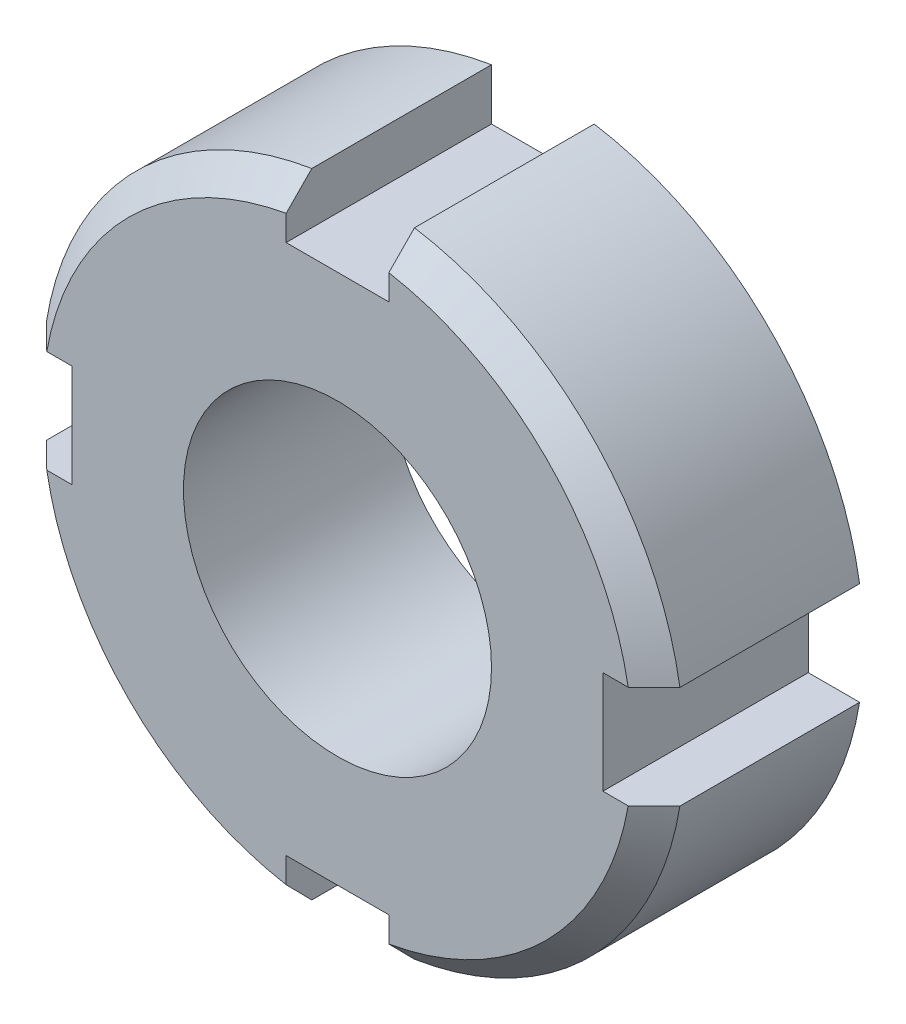
ISO-10303-21;
HEADER;
FILE_DESCRIPTION(('STEP AP214'),'2;1');
FILE_NAME('part.step','',(''),(''),'','','');
FILE_SCHEMA(('AUTOMOTIVE_DESIGN { 1 0 10303 214 1 1 1 1 }'));
ENDSEC;
DATA;
#1=APPLICATION_CONTEXT('core data for automotive mechanical design processes');
#2=APPLICATION_PROTOCOL_DEFINITION('international standard','automotive_design',2000,#1);
#3=PRODUCT_CONTEXT('',#1,'mechanical');
#4=PRODUCT('Part','Part','',(#3));
#5=PRODUCT_RELATED_PRODUCT_CATEGORY('part','',(#4));
#6=PRODUCT_DEFINITION_FORMATION('','',#4);
#7=PRODUCT_DEFINITION_CONTEXT('part definition',#1,'design');
#8=PRODUCT_DEFINITION('design','',#6,#7);
#9=PRODUCT_DEFINITION_SHAPE('','',#8);
#10=(LENGTH_UNIT() NAMED_UNIT(*) SI_UNIT(.MILLI.,.METRE.));
#11=(NAMED_UNIT(*) PLANE_ANGLE_UNIT() SI_UNIT($,.RADIAN.));
#12=(NAMED_UNIT(*) SI_UNIT($,.STERADIAN.) SOLID_ANGLE_UNIT());
#13=UNCERTAINTY_MEASURE_WITH_UNIT(LENGTH_MEASURE(1.E-05),#10,'distance_accuracy_value','');
#14=(GEOMETRIC_REPRESENTATION_CONTEXT(3) GLOBAL_UNCERTAINTY_ASSIGNED_CONTEXT((#13)) GLOBAL_UNIT_ASSIGNED_CONTEXT((#10,
#11,#12)) REPRESENTATION_CONTEXT('',''));
#15=CARTESIAN_POINT('',(0.,0.,0.));
#16=DIRECTION('',(0.,0.,1.));
#17=DIRECTION('',(1.,0.,0.));
#18=AXIS2_PLACEMENT_3D('',#15,#16,#17);
#19=CARTESIAN_POINT('',(-2.,10.3389626792531,4.));
#20=DIRECTION('',(0.,-1.,0.));
#21=DIRECTION('',(0.,0.,-1.));
#22=AXIS2_PLACEMENT_3D('',#19,#20,#21);
#23=PLANE('',#22);
#24=DIRECTION('',(-1.,0.,0.));
#25=VECTOR('',#24,1.);
#26=CARTESIAN_POINT('',(-2.,10.3389626792531,-4.));
#27=LINE('',#26,#25);
#28=CARTESIAN_POINT('',(2.,10.3389626792531,-4.));
#29=VERTEX_POINT('',#28);
#30=CARTESIAN_POINT('',(-2.,10.3389626792531,-4.));
#31=VERTEX_POINT('',#30);
#32=EDGE_CURVE('E211',#29,#31,#27,.T.);
#33=ORIENTED_EDGE('',*,*,#32,.T.);
#34=DIRECTION('',(0.,0.,-1.));
#35=VECTOR('',#34,1.);
#36=CARTESIAN_POINT('',(-2.,10.3389626792531,4.));
#37=LINE('',#36,#35);
#38=CARTESIAN_POINT('',(-2.,10.3389626792531,4.));
#39=VERTEX_POINT('',#38);
#40=EDGE_CURVE('E194',#39,#31,#37,.T.);
#41=ORIENTED_EDGE('',*,*,#40,.F.);
#42=DIRECTION('',(-1.,0.,0.));
#43=VECTOR('',#42,1.);
#44=CARTESIAN_POINT('',(-2.,10.3389626792531,4.));
#45=LINE('',#44,#43);
#46=CARTESIAN_POINT('',(2.,10.3389626792531,4.));
#47=VERTEX_POINT('',#46);
#48=EDGE_CURVE('E202',#47,#39,#45,.T.);
#49=ORIENTED_EDGE('',*,*,#48,.F.);
#50=DIRECTION('',(0.,0.,-1.));
#51=VECTOR('',#50,1.);
#52=CARTESIAN_POINT('',(2.,10.3389626792531,4.));
#53=LINE('',#52,#51);
#54=EDGE_CURVE('E518',#47,#29,#53,.T.);
#55=ORIENTED_EDGE('',*,*,#54,.T.);
#56=EDGE_LOOP('',(#33,#41,#49,#55));
#57=FACE_BOUND('',#56,.T.);
#58=ADVANCED_FACE('F44',(#57),#23,.F.);
#59=CARTESIAN_POINT('',(-2.,12.3389626792531,4.));
#60=DIRECTION('',(-1.,0.,0.));
#61=DIRECTION('',(0.,-1.,0.));
#62=AXIS2_PLACEMENT_3D('',#59,#60,#61);
#63=PLANE('',#62);
#64=DIRECTION('',(0.,0.,-1.));
#65=VECTOR('',#64,1.);
#66=CARTESIAN_POINT('',(-2.,12.3389626792531,4.));
#67=LINE('',#66,#65);
#68=CARTESIAN_POINT('',(-2.,12.3389626792531,3.));
#69=VERTEX_POINT('',#68);
#70=CARTESIAN_POINT('',(-2.,12.3389626792531,-4.));
#71=VERTEX_POINT('',#70);
#72=EDGE_CURVE('E217',#69,#71,#67,.T.);
#73=ORIENTED_EDGE('',*,*,#72,.F.);
#74=CARTESIAN_POINT('',(-2.,12.3389626792531,3.));
#75=CARTESIAN_POINT('',(-2.,12.1700268878536,3.1667674573597));
#76=CARTESIAN_POINT('',(-2.,12.0010414069381,3.33348451906443));
#77=CARTESIAN_POINT('',(-2.,11.6629710648232,3.66681785239852));
#78=CARTESIAN_POINT('',(-2.,11.493886203623,3.83343412402712));
#79=CARTESIAN_POINT('',(-2.,11.3247516529061,4.));
#80=B_SPLINE_CURVE_WITH_KNOTS('',3,(#74,#75,#76,#77,#78,#79),.UNSPECIFIED.,.F.,.F.,(4,2,4),(0.,
0.712148890902168,1.42429778707946),.UNSPECIFIED.);
#81=CARTESIAN_POINT('',(-2.,11.3247516529061,4.));
#82=VERTEX_POINT('',#81);
#83=EDGE_CURVE('E197',#69,#82,#80,.T.);
#84=ORIENTED_EDGE('',*,*,#83,.T.);
#85=DIRECTION('',(0.,1.,0.));
#86=VECTOR('',#85,1.);
#87=CARTESIAN_POINT('',(-2.,12.3389626792531,4.));
#88=LINE('',#87,#86);
#89=EDGE_CURVE('E190',#39,#82,#88,.T.);
#90=ORIENTED_EDGE('',*,*,#89,.F.);
#91=ORIENTED_EDGE('',*,*,#40,.T.);
#92=DIRECTION('',(0.,1.,0.));
#93=VECTOR('',#92,1.);
#94=CARTESIAN_POINT('',(-2.,12.3389626792531,-4.));
#95=LINE('',#94,#93);
#96=EDGE_CURVE('E530',#31,#71,#95,.T.);
#97=ORIENTED_EDGE('',*,*,#96,.T.);
#98=EDGE_LOOP('',(#73,#84,#90,#91,#97));
#99=FACE_BOUND('',#98,.T.);
#100=ADVANCED_FACE('F188',(#99),#63,.F.);
#101=CARTESIAN_POINT('',(0.,0.,4.));
#102=DIRECTION('',(0.,0.,-1.));
#103=DIRECTION('',(-1.,0.,0.));
#104=AXIS2_PLACEMENT_3D('',#101,#102,#103);
#105=CYLINDRICAL_SURFACE('',#104,12.5);
#106=DIRECTION('',(0.,0.,-1.));
#107=VECTOR('',#106,1.);
#108=CARTESIAN_POINT('',(-12.3389626792531,2.,4.));
#109=LINE('',#108,#107);
#110=CARTESIAN_POINT('',(-12.3389626792531,2.,3.));
#111=VERTEX_POINT('',#110);
#112=CARTESIAN_POINT('',(-12.3389626792531,2.,-4.));
#113=VERTEX_POINT('',#112);
#114=EDGE_CURVE('E218',#111,#113,#109,.T.);
#115=ORIENTED_EDGE('',*,*,#114,.F.);
#116=CARTESIAN_POINT('',(0.,0.,3.));
#117=DIRECTION('',(0.,0.,1.));
#118=DIRECTION('',(1.,0.,0.));
#119=AXIS2_PLACEMENT_3D('',#116,#117,#118);
#120=CIRCLE('',#119,12.5);
#121=EDGE_CURVE('E307',#111,#69,#120,.F.);
#122=ORIENTED_EDGE('',*,*,#121,.T.);
#123=ORIENTED_EDGE('',*,*,#72,.T.);
#124=CARTESIAN_POINT('',(0.,0.,-4.));
#125=DIRECTION('',(0.,0.,1.));
#126=DIRECTION('',(1.,0.,0.));
#127=AXIS2_PLACEMENT_3D('',#124,#125,#126);
#128=CIRCLE('',#127,12.5);
#129=EDGE_CURVE('E526',#71,#113,#128,.T.);
#130=ORIENTED_EDGE('',*,*,#129,.T.);
#131=EDGE_LOOP('',(#115,#122,#123,#130));
#132=FACE_BOUND('',#131,.T.);
#133=ADVANCED_FACE('F319',(#132),#105,.T.);
#134=CARTESIAN_POINT('',(-12.3389626792531,2.,4.));
#135=DIRECTION('',(0.,1.,0.));
#136=DIRECTION('',(-1.,0.,0.));
#137=AXIS2_PLACEMENT_3D('',#134,#135,#136);
#138=PLANE('',#137);
#139=DIRECTION('',(1.,0.,0.));
#140=VECTOR('',#139,1.);
#141=CARTESIAN_POINT('',(-12.3389626792531,2.,4.));
#142=LINE('',#141,#140);
#143=CARTESIAN_POINT('',(-11.3247516529061,2.,4.));
#144=VERTEX_POINT('',#143);
#145=CARTESIAN_POINT('',(-10.3389626792531,2.,4.));
#146=VERTEX_POINT('',#145);
#147=EDGE_CURVE('E198',#144,#146,#142,.T.);
#148=ORIENTED_EDGE('',*,*,#147,.F.);
#149=CARTESIAN_POINT('',(-11.3247516529061,2.,4.));
#150=CARTESIAN_POINT('',(-11.493886203623,2.,3.83343412402712));
#151=CARTESIAN_POINT('',(-11.6629710648232,2.,3.66681785239852));
#152=CARTESIAN_POINT('',(-12.0010414069381,2.,3.33348451906444));
#153=CARTESIAN_POINT('',(-12.1700268878536,2.,3.1667674573597));
#154=CARTESIAN_POINT('',(-12.3389626792531,2.,3.));
#155=B_SPLINE_CURVE_WITH_KNOTS('',3,(#149,#150,#151,#152,#153,#154),.UNSPECIFIED.,.F.,.F.,(4,2,
4),(0.,0.71214889617729,1.42429778707946),.UNSPECIFIED.);
#156=EDGE_CURVE('E303',#144,#111,#155,.T.);
#157=ORIENTED_EDGE('',*,*,#156,.T.);
#158=ORIENTED_EDGE('',*,*,#114,.T.);
#159=DIRECTION('',(1.,0.,0.));
#160=VECTOR('',#159,1.);
#161=CARTESIAN_POINT('',(-12.3389626792531,2.,-4.));
#162=LINE('',#161,#160);
#163=CARTESIAN_POINT('',(-10.3389626792531,2.,-4.));
#164=VERTEX_POINT('',#163);
#165=EDGE_CURVE('E531',#113,#164,#162,.T.);
#166=ORIENTED_EDGE('',*,*,#165,.T.);
#167=DIRECTION('',(0.,0.,-1.));
#168=VECTOR('',#167,1.);
#169=CARTESIAN_POINT('',(-10.3389626792531,2.,4.));
#170=LINE('',#169,#168);
#171=EDGE_CURVE('E586',#146,#164,#170,.T.);
#172=ORIENTED_EDGE('',*,*,#171,.F.);
#173=EDGE_LOOP('',(#148,#157,#158,#166,#172));
#174=FACE_BOUND('',#173,.T.);
#175=ADVANCED_FACE('F313',(#174),#138,.F.);
#176=CARTESIAN_POINT('',(-10.3389626792531,-2.,4.));
#177=DIRECTION('',(1.,0.,0.));
#178=DIRECTION('',(0.,0.,-1.));
#179=AXIS2_PLACEMENT_3D('',#176,#177,#178);
#180=PLANE('',#179);
#181=DIRECTION('',(0.,-1.,0.));
#182=VECTOR('',#181,1.);
#183=CARTESIAN_POINT('',(-10.3389626792531,-2.,-4.));
#184=LINE('',#183,#182);
#185=CARTESIAN_POINT('',(-10.3389626792531,-2.,-4.));
#186=VERTEX_POINT('',#185);
#187=EDGE_CURVE('E533',#164,#186,#184,.T.);
#188=ORIENTED_EDGE('',*,*,#187,.T.);
#189=DIRECTION('',(0.,0.,-1.));
#190=VECTOR('',#189,1.);
#191=CARTESIAN_POINT('',(-10.3389626792531,-2.,4.));
#192=LINE('',#191,#190);
#193=CARTESIAN_POINT('',(-10.3389626792531,-2.,4.));
#194=VERTEX_POINT('',#193);
#195=EDGE_CURVE('E587',#194,#186,#192,.T.);
#196=ORIENTED_EDGE('',*,*,#195,.F.);
#197=DIRECTION('',(0.,-1.,0.));
#198=VECTOR('',#197,1.);
#199=CARTESIAN_POINT('',(-10.3389626792531,-2.,4.));
#200=LINE('',#199,#198);
#201=EDGE_CURVE('E608',#146,#194,#200,.T.);
#202=ORIENTED_EDGE('',*,*,#201,.F.);
#203=ORIENTED_EDGE('',*,*,#171,.T.);
#204=EDGE_LOOP('',(#188,#196,#202,#203));
#205=FACE_BOUND('',#204,.T.);
#206=ADVANCED_FACE('F295',(#205),#180,.F.);
#207=CARTESIAN_POINT('',(-12.3389626792531,-2.,4.));
#208=DIRECTION('',(0.,-1.,0.));
#209=DIRECTION('',(1.,0.,0.));
#210=AXIS2_PLACEMENT_3D('',#207,#208,#209);
#211=PLANE('',#210);
#212=DIRECTION('',(0.,0.,-1.));
#213=VECTOR('',#212,1.);
#214=CARTESIAN_POINT('',(-12.3389626792531,-2.,4.));
#215=LINE('',#214,#213);
#216=CARTESIAN_POINT('',(-12.3389626792531,-2.,3.));
#217=VERTEX_POINT('',#216);
#218=CARTESIAN_POINT('',(-12.3389626792531,-2.,-4.));
#219=VERTEX_POINT('',#218);
#220=EDGE_CURVE('E581',#217,#219,#215,.T.);
#221=ORIENTED_EDGE('',*,*,#220,.F.);
#222=CARTESIAN_POINT('',(-12.3389626792531,-2.,3.));
#223=CARTESIAN_POINT('',(-12.1700268878536,-2.,3.1667674573597));
#224=CARTESIAN_POINT('',(-12.0010414069381,-2.,3.33348451906444));
#225=CARTESIAN_POINT('',(-11.6629710648232,-2.,3.66681785239852));
#226=CARTESIAN_POINT('',(-11.493886203623,-2.,3.83343412402712));
#227=CARTESIAN_POINT('',(-11.3247516529061,-2.,4.));
#228=B_SPLINE_CURVE_WITH_KNOTS('',3,(#222,#223,#224,#225,#226,#227),.UNSPECIFIED.,.F.,.F.,(4,2,
4),(0.,0.712148890902172,1.42429778707946),.UNSPECIFIED.);
#229=CARTESIAN_POINT('',(-11.3247516529061,-2.,4.));
#230=VERTEX_POINT('',#229);
#231=EDGE_CURVE('E300',#217,#230,#228,.T.);
#232=ORIENTED_EDGE('',*,*,#231,.T.);
#233=DIRECTION('',(-1.,0.,0.));
#234=VECTOR('',#233,1.);
#235=CARTESIAN_POINT('',(-12.3389626792531,-2.,4.));
#236=LINE('',#235,#234);
#237=EDGE_CURVE('E607',#194,#230,#236,.T.);
#238=ORIENTED_EDGE('',*,*,#237,.F.);
#239=ORIENTED_EDGE('',*,*,#195,.T.);
#240=DIRECTION('',(-1.,0.,0.));
#241=VECTOR('',#240,1.);
#242=CARTESIAN_POINT('',(-12.3389626792531,-2.,-4.));
#243=LINE('',#242,#241);
#244=EDGE_CURVE('E540',#186,#219,#243,.T.);
#245=ORIENTED_EDGE('',*,*,#244,.T.);
#246=EDGE_LOOP('',(#221,#232,#238,#239,#245));
#247=FACE_BOUND('',#246,.T.);
#248=ADVANCED_FACE('F289',(#247),#211,.F.);
#249=CARTESIAN_POINT('',(0.,0.,4.));
#250=DIRECTION('',(0.,0.,-1.));
#251=DIRECTION('',(-1.,0.,0.));
#252=AXIS2_PLACEMENT_3D('',#249,#250,#251);
#253=CYLINDRICAL_SURFACE('',#252,12.5);
#254=DIRECTION('',(0.,0.,-1.));
#255=VECTOR('',#254,1.);
#256=CARTESIAN_POINT('',(-2.,-12.3389626792531,4.));
#257=LINE('',#256,#255);
#258=CARTESIAN_POINT('',(-2.,-12.3389626792531,3.));
#259=VERTEX_POINT('',#258);
#260=CARTESIAN_POINT('',(-2.,-12.3389626792531,-4.));
#261=VERTEX_POINT('',#260);
#262=EDGE_CURVE('E585',#259,#261,#257,.T.);
#263=ORIENTED_EDGE('',*,*,#262,.F.);
#264=CARTESIAN_POINT('',(0.,0.,3.));
#265=DIRECTION('',(0.,0.,1.));
#266=DIRECTION('',(1.,0.,0.));
#267=AXIS2_PLACEMENT_3D('',#264,#265,#266);
#268=CIRCLE('',#267,12.5);
#269=EDGE_CURVE('E277',#259,#217,#268,.F.);
#270=ORIENTED_EDGE('',*,*,#269,.T.);
#271=ORIENTED_EDGE('',*,*,#220,.T.);
#272=CARTESIAN_POINT('',(0.,0.,-4.));
#273=DIRECTION('',(0.,0.,1.));
#274=DIRECTION('',(1.,0.,0.));
#275=AXIS2_PLACEMENT_3D('',#272,#273,#274);
#276=CIRCLE('',#275,12.5);
#277=EDGE_CURVE('E538',#219,#261,#276,.T.);
#278=ORIENTED_EDGE('',*,*,#277,.T.);
#279=EDGE_LOOP('',(#263,#270,#271,#278));
#280=FACE_BOUND('',#279,.T.);
#281=ADVANCED_FACE('F283',(#280),#253,.T.);
#282=CARTESIAN_POINT('',(-2.,-12.3389626792531,4.));
#283=DIRECTION('',(-1.,0.,0.));
#284=DIRECTION('',(0.,0.,1.));
#285=AXIS2_PLACEMENT_3D('',#282,#283,#284);
#286=PLANE('',#285);
#287=DIRECTION('',(0.,1.,0.));
#288=VECTOR('',#287,1.);
#289=CARTESIAN_POINT('',(-2.,-12.3389626792531,4.));
#290=LINE('',#289,#288);
#291=CARTESIAN_POINT('',(-2.,-11.3247516529061,4.));
#292=VERTEX_POINT('',#291);
#293=CARTESIAN_POINT('',(-2.,-10.3389626792531,4.));
#294=VERTEX_POINT('',#293);
#295=EDGE_CURVE('E606',#292,#294,#290,.T.);
#296=ORIENTED_EDGE('',*,*,#295,.F.);
#297=CARTESIAN_POINT('',(-2.,-11.3247516529061,4.));
#298=CARTESIAN_POINT('',(-2.,-11.493886203623,3.83343412402712));
#299=CARTESIAN_POINT('',(-2.,-11.6629710648232,3.66681785239852));
#300=CARTESIAN_POINT('',(-2.,-12.0010414069381,3.33348451906444));
#301=CARTESIAN_POINT('',(-2.,-12.1700268878536,3.1667674573597));
#302=CARTESIAN_POINT('',(-2.,-12.3389626792531,3.));
#303=B_SPLINE_CURVE_WITH_KNOTS('',3,(#297,#298,#299,#300,#301,#302),.UNSPECIFIED.,.F.,.F.,(4,2,
4),(0.,0.712148896177292,1.42429778707946),.UNSPECIFIED.);
#304=EDGE_CURVE('E266',#292,#259,#303,.T.);
#305=ORIENTED_EDGE('',*,*,#304,.T.);
#306=ORIENTED_EDGE('',*,*,#262,.T.);
#307=DIRECTION('',(0.,1.,0.));
#308=VECTOR('',#307,1.);
#309=CARTESIAN_POINT('',(-2.,-12.3389626792531,-4.));
#310=LINE('',#309,#308);
#311=CARTESIAN_POINT('',(-2.,-10.3389626792531,-4.));
#312=VERTEX_POINT('',#311);
#313=EDGE_CURVE('E545',#261,#312,#310,.T.);
#314=ORIENTED_EDGE('',*,*,#313,.T.);
#315=DIRECTION('',(0.,0.,-1.));
#316=VECTOR('',#315,1.);
#317=CARTESIAN_POINT('',(-2.,-10.3389626792531,4.));
#318=LINE('',#317,#316);
#319=EDGE_CURVE('E576',#294,#312,#318,.T.);
#320=ORIENTED_EDGE('',*,*,#319,.F.);
#321=EDGE_LOOP('',(#296,#305,#306,#314,#320));
#322=FACE_BOUND('',#321,.T.);
#323=ADVANCED_FACE('F282',(#322),#286,.F.);
#324=CARTESIAN_POINT('',(2.,-10.3389626792531,4.));
#325=DIRECTION('',(0.,1.,0.));
#326=DIRECTION('',(0.,0.,1.));
#327=AXIS2_PLACEMENT_3D('',#324,#325,#326);
#328=PLANE('',#327);
#329=DIRECTION('',(1.,0.,0.));
#330=VECTOR('',#329,1.);
#331=CARTESIAN_POINT('',(2.,-10.3389626792531,-4.));
#332=LINE('',#331,#330);
#333=CARTESIAN_POINT('',(2.,-10.3389626792531,-4.));
#334=VERTEX_POINT('',#333);
#335=EDGE_CURVE('E543',#312,#334,#332,.T.);
#336=ORIENTED_EDGE('',*,*,#335,.T.);
#337=DIRECTION('',(0.,0.,-1.));
#338=VECTOR('',#337,1.);
#339=CARTESIAN_POINT('',(2.,-10.3389626792531,4.));
#340=LINE('',#339,#338);
#341=CARTESIAN_POINT('',(2.,-10.3389626792531,4.));
#342=VERTEX_POINT('',#341);
#343=EDGE_CURVE('E577',#342,#334,#340,.T.);
#344=ORIENTED_EDGE('',*,*,#343,.F.);
#345=DIRECTION('',(1.,0.,0.));
#346=VECTOR('',#345,1.);
#347=CARTESIAN_POINT('',(2.,-10.3389626792531,4.));
#348=LINE('',#347,#346);
#349=EDGE_CURVE('E615',#294,#342,#348,.T.);
#350=ORIENTED_EDGE('',*,*,#349,.F.);
#351=ORIENTED_EDGE('',*,*,#319,.T.);
#352=EDGE_LOOP('',(#336,#344,#350,#351));
#353=FACE_BOUND('',#352,.T.);
#354=ADVANCED_FACE('F262',(#353),#328,.F.);
#355=CARTESIAN_POINT('',(2.,-12.3389626792531,4.));
#356=DIRECTION('',(1.,0.,0.));
#357=DIRECTION('',(0.,1.,0.));
#358=AXIS2_PLACEMENT_3D('',#355,#356,#357);
#359=PLANE('',#358);
#360=DIRECTION('',(0.,0.,-1.));
#361=VECTOR('',#360,1.);
#362=CARTESIAN_POINT('',(2.,-12.3389626792531,4.));
#363=LINE('',#362,#361);
#364=CARTESIAN_POINT('',(2.,-12.3389626792531,3.));
#365=VERTEX_POINT('',#364);
#366=CARTESIAN_POINT('',(2.,-12.3389626792531,-4.));
#367=VERTEX_POINT('',#366);
#368=EDGE_CURVE('E573',#365,#367,#363,.T.);
#369=ORIENTED_EDGE('',*,*,#368,.F.);
#370=CARTESIAN_POINT('',(2.,-12.3389626792531,3.));
#371=CARTESIAN_POINT('',(2.,-12.1700268878536,3.1667674573597));
#372=CARTESIAN_POINT('',(2.,-12.0010414069381,3.33348451906444));
#373=CARTESIAN_POINT('',(2.,-11.6629710648232,3.66681785239852));
#374=CARTESIAN_POINT('',(2.,-11.493886203623,3.83343412402712));
#375=CARTESIAN_POINT('',(2.,-11.3247516529061,4.));
#376=B_SPLINE_CURVE_WITH_KNOTS('',3,(#370,#371,#372,#373,#374,#375),.UNSPECIFIED.,.F.,.F.,(4,2,
4),(0.,0.712148890902171,1.42429778707946),.UNSPECIFIED.);
#377=CARTESIAN_POINT('',(2.,-11.3247516529061,4.));
#378=VERTEX_POINT('',#377);
#379=EDGE_CURVE('E261',#365,#378,#376,.T.);
#380=ORIENTED_EDGE('',*,*,#379,.T.);
#381=DIRECTION('',(0.,-1.,0.));
#382=VECTOR('',#381,1.);
#383=CARTESIAN_POINT('',(2.,-12.3389626792531,4.));
#384=LINE('',#383,#382);
#385=EDGE_CURVE('E616',#342,#378,#384,.T.);
#386=ORIENTED_EDGE('',*,*,#385,.F.);
#387=ORIENTED_EDGE('',*,*,#343,.T.);
#388=DIRECTION('',(0.,-1.,0.));
#389=VECTOR('',#388,1.);
#390=CARTESIAN_POINT('',(2.,-12.3389626792531,-4.));
#391=LINE('',#390,#389);
#392=EDGE_CURVE('E550',#334,#367,#391,.T.);
#393=ORIENTED_EDGE('',*,*,#392,.T.);
#394=EDGE_LOOP('',(#369,#380,#386,#387,#393));
#395=FACE_BOUND('',#394,.T.);
#396=ADVANCED_FACE('F257',(#395),#359,.F.);
#397=CARTESIAN_POINT('',(0.,0.,4.));
#398=DIRECTION('',(0.,0.,-1.));
#399=DIRECTION('',(-1.,0.,0.));
#400=AXIS2_PLACEMENT_3D('',#397,#398,#399);
#401=CYLINDRICAL_SURFACE('',#400,12.5);
#402=DIRECTION('',(0.,0.,-1.));
#403=VECTOR('',#402,1.);
#404=CARTESIAN_POINT('',(12.3389626792531,-2.00000000000001,4.));
#405=LINE('',#404,#403);
#406=CARTESIAN_POINT('',(12.3389626792531,-2.00000000000001,3.));
#407=VERTEX_POINT('',#406);
#408=CARTESIAN_POINT('',(12.3389626792531,-2.00000000000001,-4.));
#409=VERTEX_POINT('',#408);
#410=EDGE_CURVE('E575',#407,#409,#405,.T.);
#411=ORIENTED_EDGE('',*,*,#410,.F.);
#412=CARTESIAN_POINT('',(0.,0.,3.));
#413=DIRECTION('',(0.,0.,1.));
#414=DIRECTION('',(1.,0.,0.));
#415=AXIS2_PLACEMENT_3D('',#412,#413,#414);
#416=CIRCLE('',#415,12.5);
#417=EDGE_CURVE('E237',#407,#365,#416,.F.);
#418=ORIENTED_EDGE('',*,*,#417,.T.);
#419=ORIENTED_EDGE('',*,*,#368,.T.);
#420=CARTESIAN_POINT('',(0.,0.,-4.));
#421=DIRECTION('',(0.,0.,1.));
#422=DIRECTION('',(1.,0.,0.));
#423=AXIS2_PLACEMENT_3D('',#420,#421,#422);
#424=CIRCLE('',#423,12.5);
#425=EDGE_CURVE('E546',#367,#409,#424,.T.);
#426=ORIENTED_EDGE('',*,*,#425,.T.);
#427=EDGE_LOOP('',(#411,#418,#419,#426));
#428=FACE_BOUND('',#427,.T.);
#429=ADVANCED_FACE('F255',(#428),#401,.T.);
#430=CARTESIAN_POINT('',(12.3389626792531,-2.,4.));
#431=DIRECTION('',(0.,-1.,0.));
#432=DIRECTION('',(1.,0.,0.));
#433=AXIS2_PLACEMENT_3D('',#430,#431,#432);
#434=PLANE('',#433);
#435=DIRECTION('',(-1.,0.,0.));
#436=VECTOR('',#435,1.);
#437=CARTESIAN_POINT('',(12.3389626792531,-2.,4.));
#438=LINE('',#437,#436);
#439=CARTESIAN_POINT('',(11.3247516529061,-2.,4.));
#440=VERTEX_POINT('',#439);
#441=CARTESIAN_POINT('',(10.3389626792531,-2.,4.));
#442=VERTEX_POINT('',#441);
#443=EDGE_CURVE('E524',#440,#442,#438,.T.);
#444=ORIENTED_EDGE('',*,*,#443,.F.);
#445=CARTESIAN_POINT('',(11.3247516529061,-2.,4.));
#446=CARTESIAN_POINT('',(11.493886203623,-2.,3.83343412402712));
#447=CARTESIAN_POINT('',(11.6629710648232,-2.,3.66681785239852));
#448=CARTESIAN_POINT('',(12.0010414069381,-2.,3.33348451906444));
#449=CARTESIAN_POINT('',(12.1700268878536,-2.,3.1667674573597));
#450=CARTESIAN_POINT('',(12.3389626792531,-2.,3.));
#451=B_SPLINE_CURVE_WITH_KNOTS('',3,(#445,#446,#447,#448,#449,#450),.UNSPECIFIED.,.F.,.F.,(4,2,
4),(0.,0.71214889617729,1.42429778707946),.UNSPECIFIED.);
#452=EDGE_CURVE('E233',#440,#407,#451,.T.);
#453=ORIENTED_EDGE('',*,*,#452,.T.);
#454=ORIENTED_EDGE('',*,*,#410,.T.);
#455=DIRECTION('',(-1.,0.,0.));
#456=VECTOR('',#455,1.);
#457=CARTESIAN_POINT('',(12.3389626792531,-2.,-4.));
#458=LINE('',#457,#456);
#459=CARTESIAN_POINT('',(10.3389626792531,-2.,-4.));
#460=VERTEX_POINT('',#459);
#461=EDGE_CURVE('E551',#409,#460,#458,.T.);
#462=ORIENTED_EDGE('',*,*,#461,.T.);
#463=DIRECTION('',(0.,0.,-1.));
#464=VECTOR('',#463,1.);
#465=CARTESIAN_POINT('',(10.3389626792531,-2.,4.));
#466=LINE('',#465,#464);
#467=EDGE_CURVE('E567',#442,#460,#466,.T.);
#468=ORIENTED_EDGE('',*,*,#467,.F.);
#469=EDGE_LOOP('',(#444,#453,#454,#462,#468));
#470=FACE_BOUND('',#469,.T.);
#471=ADVANCED_FACE('F246',(#470),#434,.F.);
#472=CARTESIAN_POINT('',(10.3389626792531,2.,4.));
#473=DIRECTION('',(-1.,0.,0.));
#474=DIRECTION('',(0.,0.,1.));
#475=AXIS2_PLACEMENT_3D('',#472,#473,#474);
#476=PLANE('',#475);
#477=DIRECTION('',(0.,1.,0.));
#478=VECTOR('',#477,1.);
#479=CARTESIAN_POINT('',(10.3389626792531,2.,-4.));
#480=LINE('',#479,#478);
#481=CARTESIAN_POINT('',(10.3389626792531,2.,-4.));
#482=VERTEX_POINT('',#481);
#483=EDGE_CURVE('E554',#460,#482,#480,.T.);
#484=ORIENTED_EDGE('',*,*,#483,.T.);
#485=DIRECTION('',(0.,0.,-1.));
#486=VECTOR('',#485,1.);
#487=CARTESIAN_POINT('',(10.3389626792531,2.,4.));
#488=LINE('',#487,#486);
#489=CARTESIAN_POINT('',(10.3389626792531,2.,4.));
#490=VERTEX_POINT('',#489);
#491=EDGE_CURVE('E570',#490,#482,#488,.T.);
#492=ORIENTED_EDGE('',*,*,#491,.F.);
#493=DIRECTION('',(0.,1.,0.));
#494=VECTOR('',#493,1.);
#495=CARTESIAN_POINT('',(10.3389626792531,2.,4.));
#496=LINE('',#495,#494);
#497=EDGE_CURVE('E520',#442,#490,#496,.T.);
#498=ORIENTED_EDGE('',*,*,#497,.F.);
#499=ORIENTED_EDGE('',*,*,#467,.T.);
#500=EDGE_LOOP('',(#484,#492,#498,#499));
#501=FACE_BOUND('',#500,.T.);
#502=ADVANCED_FACE('F252',(#501),#476,.F.);
#503=CARTESIAN_POINT('',(12.3389626792531,2.,4.));
#504=DIRECTION('',(0.,1.,0.));
#505=DIRECTION('',(-1.,0.,0.));
#506=AXIS2_PLACEMENT_3D('',#503,#504,#505);
#507=PLANE('',#506);
#508=DIRECTION('',(0.,0.,-1.));
#509=VECTOR('',#508,1.);
#510=CARTESIAN_POINT('',(12.3389626792531,2.,4.));
#511=LINE('',#510,#509);
#512=CARTESIAN_POINT('',(12.3389626792531,2.,3.));
#513=VERTEX_POINT('',#512);
#514=CARTESIAN_POINT('',(12.3389626792531,2.,-4.));
#515=VERTEX_POINT('',#514);
#516=EDGE_CURVE('E513',#513,#515,#511,.T.);
#517=ORIENTED_EDGE('',*,*,#516,.F.);
#518=CARTESIAN_POINT('',(12.3389626792531,2.,3.));
#519=CARTESIAN_POINT('',(12.1700268878536,2.,3.1667674573597));
#520=CARTESIAN_POINT('',(12.0010414069381,2.,3.33348451906444));
#521=CARTESIAN_POINT('',(11.6629710648232,2.,3.66681785239852));
#522=CARTESIAN_POINT('',(11.493886203623,2.,3.83343412402712));
#523=CARTESIAN_POINT('',(11.3247516529061,2.,4.));
#524=B_SPLINE_CURVE_WITH_KNOTS('',3,(#518,#519,#520,#521,#522,#523),.UNSPECIFIED.,.F.,.F.,(4,2,
4),(0.,0.712148890902171,1.42429778707946),.UNSPECIFIED.);
#525=CARTESIAN_POINT('',(11.3247516529061,2.,4.));
#526=VERTEX_POINT('',#525);
#527=EDGE_CURVE('E11',#513,#526,#524,.T.);
#528=ORIENTED_EDGE('',*,*,#527,.T.);
#529=DIRECTION('',(1.,0.,0.));
#530=VECTOR('',#529,1.);
#531=CARTESIAN_POINT('',(12.3389626792531,2.,4.));
#532=LINE('',#531,#530);
#533=EDGE_CURVE('E514',#490,#526,#532,.T.);
#534=ORIENTED_EDGE('',*,*,#533,.F.);
#535=ORIENTED_EDGE('',*,*,#491,.T.);
#536=DIRECTION('',(1.,0.,0.));
#537=VECTOR('',#536,1.);
#538=CARTESIAN_POINT('',(12.3389626792531,2.,-4.));
#539=LINE('',#538,#537);
#540=EDGE_CURVE('E560',#482,#515,#539,.T.);
#541=ORIENTED_EDGE('',*,*,#540,.T.);
#542=EDGE_LOOP('',(#517,#528,#534,#535,#541));
#543=FACE_BOUND('',#542,.T.);
#544=ADVANCED_FACE('F341',(#543),#507,.F.);
#545=CARTESIAN_POINT('',(0.,0.,4.));
#546=DIRECTION('',(0.,0.,-1.));
#547=DIRECTION('',(-1.,0.,0.));
#548=AXIS2_PLACEMENT_3D('',#545,#546,#547);
#549=CYLINDRICAL_SURFACE('',#548,12.5);
#550=DIRECTION('',(0.,0.,-1.));
#551=VECTOR('',#550,1.);
#552=CARTESIAN_POINT('',(2.,12.3389626792531,4.));
#553=LINE('',#552,#551);
#554=CARTESIAN_POINT('',(2.,12.3389626792531,3.));
#555=VERTEX_POINT('',#554);
#556=CARTESIAN_POINT('',(2.,12.3389626792531,-4.));
#557=VERTEX_POINT('',#556);
#558=EDGE_CURVE('E562',#555,#557,#553,.T.);
#559=ORIENTED_EDGE('',*,*,#558,.F.);
#560=CARTESIAN_POINT('',(0.,0.,3.));
#561=DIRECTION('',(0.,0.,1.));
#562=DIRECTION('',(1.,0.,0.));
#563=AXIS2_PLACEMENT_3D('',#560,#561,#562);
#564=CIRCLE('',#563,12.5);
#565=EDGE_CURVE('E58',#555,#513,#564,.F.);
#566=ORIENTED_EDGE('',*,*,#565,.T.);
#567=ORIENTED_EDGE('',*,*,#516,.T.);
#568=CARTESIAN_POINT('',(0.,0.,-4.));
#569=DIRECTION('',(0.,0.,1.));
#570=DIRECTION('',(1.,0.,0.));
#571=AXIS2_PLACEMENT_3D('',#568,#569,#570);
#572=CIRCLE('',#571,12.5);
#573=EDGE_CURVE('E559',#515,#557,#572,.T.);
#574=ORIENTED_EDGE('',*,*,#573,.T.);
#575=EDGE_LOOP('',(#559,#566,#567,#574));
#576=FACE_BOUND('',#575,.T.);
#577=ADVANCED_FACE('F338',(#576),#549,.T.);
#578=CARTESIAN_POINT('',(2.,12.3389626792531,4.));
#579=DIRECTION('',(1.,0.,0.));
#580=DIRECTION('',(0.,1.,0.));
#581=AXIS2_PLACEMENT_3D('',#578,#579,#580);
#582=PLANE('',#581);
#583=DIRECTION('',(0.,-1.,0.));
#584=VECTOR('',#583,1.);
#585=CARTESIAN_POINT('',(2.,12.3389626792531,4.));
#586=LINE('',#585,#584);
#587=CARTESIAN_POINT('',(2.,11.3247516529061,4.));
#588=VERTEX_POINT('',#587);
#589=EDGE_CURVE('E210',#588,#47,#586,.T.);
#590=ORIENTED_EDGE('',*,*,#589,.F.);
#591=CARTESIAN_POINT('',(2.,11.3247516529061,4.));
#592=CARTESIAN_POINT('',(2.,11.493886203623,3.83343412402712));
#593=CARTESIAN_POINT('',(2.,11.6629710648232,3.66681785239852));
#594=CARTESIAN_POINT('',(2.,12.0010414069381,3.33348451906444));
#595=CARTESIAN_POINT('',(2.,12.1700268878536,3.1667674573597));
#596=CARTESIAN_POINT('',(2.,12.3389626792531,3.));
#597=B_SPLINE_CURVE_WITH_KNOTS('',3,(#591,#592,#593,#594,#595,#596),.UNSPECIFIED.,.F.,.F.,(4,2,
4),(0.,0.712148896177289,1.42429778707946),.UNSPECIFIED.);
#598=EDGE_CURVE('E74',#588,#555,#597,.T.);
#599=ORIENTED_EDGE('',*,*,#598,.T.);
#600=ORIENTED_EDGE('',*,*,#558,.T.);
#601=DIRECTION('',(0.,-1.,0.));
#602=VECTOR('',#601,1.);
#603=CARTESIAN_POINT('',(2.,12.3389626792531,-4.));
#604=LINE('',#603,#602);
#605=EDGE_CURVE('E212',#557,#29,#604,.T.);
#606=ORIENTED_EDGE('',*,*,#605,.T.);
#607=ORIENTED_EDGE('',*,*,#54,.F.);
#608=EDGE_LOOP('',(#590,#599,#600,#606,#607));
#609=FACE_BOUND('',#608,.T.);
#610=ADVANCED_FACE('F331',(#609),#582,.F.);
#611=CARTESIAN_POINT('',(0.,0.,4.));
#612=DIRECTION('',(0.,0.,1.));
#613=DIRECTION('',(1.,0.,0.));
#614=AXIS2_PLACEMENT_3D('',#611,#612,#613);
#615=PLANE('',#614);
#616=CARTESIAN_POINT('',(0.,0.,4.));
#617=DIRECTION('',(0.,0.,1.));
#618=DIRECTION('',(1.,0.,0.));
#619=AXIS2_PLACEMENT_3D('',#616,#617,#618);
#620=CIRCLE('',#619,6.);
#621=CARTESIAN_POINT('',(6.,0.,4.));
#622=VERTEX_POINT('',#621);
#623=EDGE_CURVE('E629',#622,#622,#620,.T.);
#624=ORIENTED_EDGE('',*,*,#623,.F.);
#625=EDGE_LOOP('',(#624));
#626=FACE_BOUND('',#625,.T.);
#627=ORIENTED_EDGE('',*,*,#385,.T.);
#628=CARTESIAN_POINT('',(0.,0.,4.));
#629=DIRECTION('',(0.,0.,1.));
#630=DIRECTION('',(1.,0.,0.));
#631=AXIS2_PLACEMENT_3D('',#628,#629,#630);
#632=CIRCLE('',#631,11.5);
#633=EDGE_CURVE('E226',#378,#440,#632,.T.);
#634=ORIENTED_EDGE('',*,*,#633,.T.);
#635=ORIENTED_EDGE('',*,*,#443,.T.);
#636=ORIENTED_EDGE('',*,*,#497,.T.);
#637=ORIENTED_EDGE('',*,*,#533,.T.);
#638=CARTESIAN_POINT('',(0.,0.,4.));
#639=DIRECTION('',(0.,0.,1.));
#640=DIRECTION('',(1.,0.,0.));
#641=AXIS2_PLACEMENT_3D('',#638,#639,#640);
#642=CIRCLE('',#641,11.5);
#643=EDGE_CURVE('E213',#526,#588,#642,.T.);
#644=ORIENTED_EDGE('',*,*,#643,.T.);
#645=ORIENTED_EDGE('',*,*,#589,.T.);
#646=ORIENTED_EDGE('',*,*,#48,.T.);
#647=ORIENTED_EDGE('',*,*,#89,.T.);
#648=CARTESIAN_POINT('',(0.,0.,4.));
#649=DIRECTION('',(0.,0.,1.));
#650=DIRECTION('',(1.,0.,0.));
#651=AXIS2_PLACEMENT_3D('',#648,#649,#650);
#652=CIRCLE('',#651,11.5);
#653=EDGE_CURVE('E220',#82,#144,#652,.T.);
#654=ORIENTED_EDGE('',*,*,#653,.T.);
#655=ORIENTED_EDGE('',*,*,#147,.T.);
#656=ORIENTED_EDGE('',*,*,#201,.T.);
#657=ORIENTED_EDGE('',*,*,#237,.T.);
#658=CARTESIAN_POINT('',(0.,0.,4.));
#659=DIRECTION('',(0.,0.,1.));
#660=DIRECTION('',(1.,0.,0.));
#661=AXIS2_PLACEMENT_3D('',#658,#659,#660);
#662=CIRCLE('',#661,11.5);
#663=EDGE_CURVE('E221',#230,#292,#662,.T.);
#664=ORIENTED_EDGE('',*,*,#663,.T.);
#665=ORIENTED_EDGE('',*,*,#295,.T.);
#666=ORIENTED_EDGE('',*,*,#349,.T.);
#667=EDGE_LOOP('',(#627,#634,#635,#636,#637,#644,#645,#646,#647,#654,#655,#656,#657,#664,#665,#666));
#668=FACE_BOUND('',#667,.T.);
#669=ADVANCED_FACE('F201',(#626,#668),#615,.T.);
#670=CARTESIAN_POINT('',(0.,0.,-4.));
#671=DIRECTION('',(0.,0.,1.));
#672=DIRECTION('',(1.,0.,0.));
#673=AXIS2_PLACEMENT_3D('',#670,#671,#672);
#674=PLANE('',#673);
#675=CARTESIAN_POINT('',(0.,0.,-4.));
#676=DIRECTION('',(0.,0.,1.));
#677=DIRECTION('',(1.,0.,0.));
#678=AXIS2_PLACEMENT_3D('',#675,#676,#677);
#679=CIRCLE('',#678,6.);
#680=CARTESIAN_POINT('',(6.,0.,-4.));
#681=VERTEX_POINT('',#680);
#682=EDGE_CURVE('E528',#681,#681,#679,.T.);
#683=ORIENTED_EDGE('',*,*,#682,.T.);
#684=EDGE_LOOP('',(#683));
#685=FACE_BOUND('',#684,.T.);
#686=ORIENTED_EDGE('',*,*,#32,.F.);
#687=ORIENTED_EDGE('',*,*,#605,.F.);
#688=ORIENTED_EDGE('',*,*,#573,.F.);
#689=ORIENTED_EDGE('',*,*,#540,.F.);
#690=ORIENTED_EDGE('',*,*,#483,.F.);
#691=ORIENTED_EDGE('',*,*,#461,.F.);
#692=ORIENTED_EDGE('',*,*,#425,.F.);
#693=ORIENTED_EDGE('',*,*,#392,.F.);
#694=ORIENTED_EDGE('',*,*,#335,.F.);
#695=ORIENTED_EDGE('',*,*,#313,.F.);
#696=ORIENTED_EDGE('',*,*,#277,.F.);
#697=ORIENTED_EDGE('',*,*,#244,.F.);
#698=ORIENTED_EDGE('',*,*,#187,.F.);
#699=ORIENTED_EDGE('',*,*,#165,.F.);
#700=ORIENTED_EDGE('',*,*,#129,.F.);
#701=ORIENTED_EDGE('',*,*,#96,.F.);
#702=EDGE_LOOP('',(#686,#687,#688,#689,#690,#691,#692,#693,#694,#695,#696,#697,#698,#699,#700,#701));
#703=FACE_BOUND('',#702,.T.);
#704=ADVANCED_FACE('F342',(#685,#703),#674,.F.);
#705=CARTESIAN_POINT('',(0.,0.,4.));
#706=DIRECTION('',(0.,0.,1.));
#707=DIRECTION('',(1.,0.,0.));
#708=AXIS2_PLACEMENT_3D('',#705,#706,#707);
#709=CYLINDRICAL_SURFACE('',#708,6.);
#710=ORIENTED_EDGE('',*,*,#682,.F.);
#711=EDGE_LOOP('',(#710));
#712=FACE_BOUND('',#711,.T.);
#713=ORIENTED_EDGE('',*,*,#623,.T.);
#714=EDGE_LOOP('',(#713));
#715=FACE_BOUND('',#714,.T.);
#716=ADVANCED_FACE('F390',(#712,#715),#709,.F.);
#717=CARTESIAN_POINT('',(0.,0.,4.));
#718=DIRECTION('',(0.,0.,-1.));
#719=DIRECTION('',(-1.,0.,0.));
#720=AXIS2_PLACEMENT_3D('',#717,#718,#719);
#721=CONICAL_SURFACE('',#720,11.5,0.785398163397446);
#722=ORIENTED_EDGE('',*,*,#379,.F.);
#723=ORIENTED_EDGE('',*,*,#417,.F.);
#724=ORIENTED_EDGE('',*,*,#452,.F.);
#725=ORIENTED_EDGE('',*,*,#633,.F.);
#726=EDGE_LOOP('',(#722,#723,#724,#725));
#727=FACE_BOUND('',#726,.T.);
#728=ADVANCED_FACE('F245',(#727),#721,.T.);
#729=CARTESIAN_POINT('',(0.,0.,4.));
#730=DIRECTION('',(0.,0.,-1.));
#731=DIRECTION('',(-1.,0.,0.));
#732=AXIS2_PLACEMENT_3D('',#729,#730,#731);
#733=CONICAL_SURFACE('',#732,11.5,0.785398163397447);
#734=ORIENTED_EDGE('',*,*,#231,.F.);
#735=ORIENTED_EDGE('',*,*,#269,.F.);
#736=ORIENTED_EDGE('',*,*,#304,.F.);
#737=ORIENTED_EDGE('',*,*,#663,.F.);
#738=EDGE_LOOP('',(#734,#735,#736,#737));
#739=FACE_BOUND('',#738,.T.);
#740=ADVANCED_FACE('F276',(#739),#733,.T.);
#741=CARTESIAN_POINT('',(0.,0.,4.));
#742=DIRECTION('',(0.,0.,-1.));
#743=DIRECTION('',(-1.,0.,0.));
#744=AXIS2_PLACEMENT_3D('',#741,#742,#743);
#745=CONICAL_SURFACE('',#744,11.5,0.785398163397444);
#746=ORIENTED_EDGE('',*,*,#83,.F.);
#747=ORIENTED_EDGE('',*,*,#121,.F.);
#748=ORIENTED_EDGE('',*,*,#156,.F.);
#749=ORIENTED_EDGE('',*,*,#653,.F.);
#750=EDGE_LOOP('',(#746,#747,#748,#749));
#751=FACE_BOUND('',#750,.T.);
#752=ADVANCED_FACE('F315',(#751),#745,.T.);
#753=CARTESIAN_POINT('',(0.,0.,4.));
#754=DIRECTION('',(0.,0.,-1.));
#755=DIRECTION('',(-1.,0.,0.));
#756=AXIS2_PLACEMENT_3D('',#753,#754,#755);
#757=CONICAL_SURFACE('',#756,11.5,0.785398163397446);
#758=ORIENTED_EDGE('',*,*,#527,.F.);
#759=ORIENTED_EDGE('',*,*,#565,.F.);
#760=ORIENTED_EDGE('',*,*,#598,.F.);
#761=ORIENTED_EDGE('',*,*,#643,.F.);
#762=EDGE_LOOP('',(#758,#759,#760,#761));
#763=FACE_BOUND('',#762,.T.);
#764=ADVANCED_FACE('F48',(#763),#757,.T.);
#765=CLOSED_SHELL('',(#58,#100,#133,#175,#206,#248,#281,#323,#354,#396,#429,#471,#502,#544,#577,
#610,#669,#704,#716,#728,#740,#752,#764));
#766=MANIFOLD_SOLID_BREP('B2',#765);
#767=ADVANCED_BREP_SHAPE_REPRESENTATION('',(#18,#766),#14);
#768=SHAPE_DEFINITION_REPRESENTATION(#9,#767);
ENDSEC;
END-ISO-10303-21;
